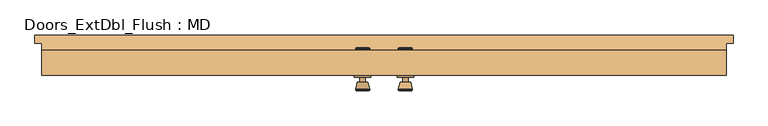
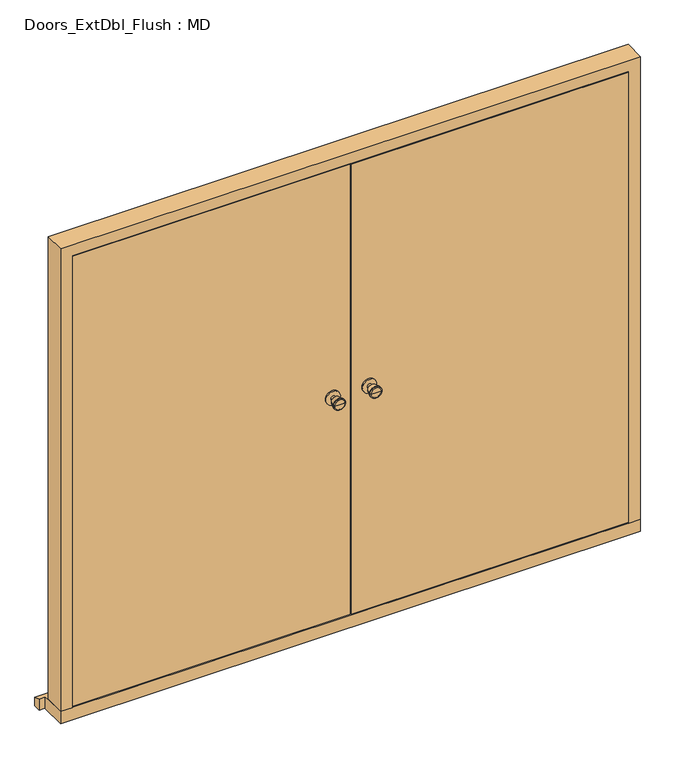
"""IFC4 building model written with IfcOpenShell, lengths in millimetres: door geometry, Doors_ExtDbl_Flush : MD."""

from ifc_helpers import new_model, si_unit, point, frame, frame_2d, origin, place, context, project, spatial, polyline, circle_curve, trimmed, segment, composite_curve, outline, extrude, faceted_brep, source, transform, mapped, element, save
from ifc_brep_helpers import plane_surface, cylinder_surface, revolved_surface, advanced_brep


def doors_extdbl_flush_md_0ef74d11(model_context):
    return source(origin(), model_context, "Body", "SolidModel", [
        advanced_brep(
        [(-76.5, -5.7, 1050.0), (-66.5, -5.7, 1050.0), (-86.5, -5.7, 1050.0), (-96.9758676, -54.7, 1050.0), (-56.0241324, -54.7, 1050.0), (-76.5, -54.7, 1050.0), (-101.5, -52.8721319, 1050.0), (-51.5, -52.8721319, 1050.0), (-101.5, -49.4084537, 1050.0), (-51.5, -49.4084537, 1050.0), (-95.136236, -24.7, 1050.0), (-57.863764, -24.7, 1050.0), (-86.5, -24.7, 1050.0), (-66.5, -24.7, 1050.0)],
        [
            (0, 1),
            (1, 2, circle_curve(frame((-76.5, -5.7, 1050.0), z_axis=(0.0, 1.0, 0.0), x_axis=(1.0, 0.0, 0.0)), 10.0)),
            (2, 0),
            (2, 1, circle_curve(frame((-76.5, -5.7, 1050.0), z_axis=(0.0, 1.0, 0.0), x_axis=(1.0, 0.0, 0.0)), 10.0)),
            (3, 4, circle_curve(frame((-76.5, -54.7, 1050.0), z_axis=(0.0, -1.0, 0.0), x_axis=(1.0, 0.0, 0.0)), 20.4758676)),
            (4, 5),
            (5, 3),
            (4, 3, circle_curve(frame((-76.5, -54.7, 1050.0), z_axis=(0.0, -1.0, 0.0), x_axis=(1.0, 0.0, 0.0)), 20.4758676)),
            (6, 7, circle_curve(frame((-76.5, -52.8721319, 1050.0), z_axis=(0.0, -1.0, 0.0), x_axis=(1.0, 0.0, 0.0)), 25.0)),
            (7, 4),
            (3, 6),
            (7, 6, circle_curve(frame((-76.5, -52.8721319, 1050.0), z_axis=(0.0, -1.0, 0.0), x_axis=(1.0, 0.0, 0.0)), 25.0)),
            (8, 9, circle_curve(frame((-76.5, -49.4084537, 1050.0), z_axis=(0.0, -1.0, 0.0), x_axis=(1.0, 0.0, 0.0)), 25.0)),
            (9, 7),
            (6, 8),
            (9, 8, circle_curve(frame((-76.5, -49.4084537, 1050.0), z_axis=(0.0, -1.0, 0.0), x_axis=(1.0, 0.0, 0.0)), 25.0)),
            (10, 11, circle_curve(frame((-76.5, -24.7, 1050.0), z_axis=(0.0, -1.0, 0.0), x_axis=(1.0, 0.0, 0.0)), 18.636236)),
            (11, 9),
            (8, 10),
            (11, 10, circle_curve(frame((-76.5, -24.7, 1050.0), z_axis=(0.0, -1.0, 0.0), x_axis=(1.0, 0.0, 0.0)), 18.636236)),
            (12, 13, circle_curve(frame((-76.5, -24.7, 1050.0), z_axis=(0.0, -1.0, 0.0), x_axis=(1.0, 0.0, 0.0)), 10.0)),
            (13, 11),
            (10, 12),
            (13, 12, circle_curve(frame((-76.5, -24.7, 1050.0), z_axis=(0.0, -1.0, 0.0), x_axis=(1.0, 0.0, 0.0)), 10.0)),
            (1, 13),
            (12, 2),
        ],
        [
            plane_surface(frame((-76.5, -5.7, 1050.0), z_axis=(0.0, 1.0, 0.0), x_axis=(1.0, 0.0, 0.0))),
            plane_surface(frame((-76.5, -54.7, 1050.0), z_axis=(0.0, -1.0, 0.0), x_axis=(1.0, 0.0, 0.0))),
            revolved_surface(polyline([(-56.0241324, -54.7, 1050.0), (-51.5, -52.8721319, 1050.0)]), (-76.5, -5.7, 1050.0), (0.0, 1.0, 0.0)),
            cylinder_surface(frame((-76.5, -5.7, 1050.0), z_axis=(0.0, 1.0, 0.0), x_axis=(1.0, 0.0, 0.0)), 25.0),
            revolved_surface(polyline([(-51.5, -49.4084537, 1050.0), (-57.863764, -24.7, 1050.0)]), (-76.5, -5.7, 1050.0), (0.0, 1.0, 0.0)),
            plane_surface(frame((-76.5, -24.7, 1050.0), z_axis=(0.0, 1.0, 0.0), x_axis=(1.0, 0.0, 0.0))),
            cylinder_surface(frame((-76.5, -5.7, 1050.0), z_axis=(0.0, 1.0, 0.0), x_axis=(1.0, 0.0, 0.0)), 10.0),
        ],
        [
            (0, [[1, 2, 3]]),
            (0, [[-3, 4, -1]]),
            (1, [[5, 6, 7]]),
            (1, [[8, -7, -6]]),
            (2, [[9, 10, -5, 11]]),
            (2, [[12, -11, -8, -10]]),
            (3, [[13, 14, -9, 15]]),
            (3, [[16, -15, -12, -14]]),
            (4, [[17, 18, -13, 19]]),
            (4, [[20, -19, -16, -18]]),
            (5, [[21, 22, -17, 23]]),
            (5, [[24, -23, -20, -22]]),
            (6, [[-2, 25, -21, 26]]),
            (6, [[-4, -26, -24, -25]]),
        ],
    ),
        extrude(outline(composite_curve([segment(trimmed(circle_curve(frame_2d((1050.0, -76.5)), 30.0), [point((1050.0, -46.5))], [point((1050.0, -106.5))], False, "CARTESIAN"), True, "CONTINUOUS"), segment(trimmed(circle_curve(frame_2d((1050.0, -76.5)), 30.0), [point((1050.0, -106.5))], [point((1050.0, -46.5))], False, "CARTESIAN"), True, "CONTINUOUS")], self_intersect=False)), frame((0.0, -5.7, 0.0), z_axis=(0.0, 1.0, 0.0), x_axis=(0.0, 0.0, 1.0)), (0.0, 0.0, 1.0), 6.0),
        advanced_brep(
        [(-76.5, 50.3, 1050.0), (-86.5, 50.3, 1050.0), (-66.5, 50.3, 1050.0), (-96.9758676, 99.3, 1050.0), (-76.5, 99.3, 1050.0), (-56.0241324, 99.3, 1050.0), (-101.5, 97.4721319, 1050.0), (-51.5, 97.4721319, 1050.0), (-101.5, 94.0084537, 1050.0), (-51.5, 94.0084537, 1050.0), (-95.136236, 69.3, 1050.0), (-57.863764, 69.3, 1050.0), (-86.5, 69.3, 1050.0), (-66.5, 69.3, 1050.0)],
        [
            (0, 1),
            (1, 2, circle_curve(frame((-76.5, 50.3, 1050.0), z_axis=(0.0, -1.0, 0.0), x_axis=(1.0, 0.0, 0.0)), 10.0)),
            (2, 0),
            (2, 1, circle_curve(frame((-76.5, 50.3, 1050.0), z_axis=(0.0, -1.0, 0.0), x_axis=(1.0, 0.0, 0.0)), 10.0)),
            (3, 4),
            (4, 5),
            (5, 3, circle_curve(frame((-76.5, 99.3, 1050.0), z_axis=(0.0, 1.0, 0.0), x_axis=(1.0, 0.0, 0.0)), 20.4758676)),
            (3, 5, circle_curve(frame((-76.5, 99.3, 1050.0), z_axis=(0.0, 1.0, 0.0), x_axis=(1.0, 0.0, 0.0)), 20.4758676)),
            (6, 3),
            (5, 7),
            (7, 6, circle_curve(frame((-76.5, 97.4721319, 1050.0), z_axis=(0.0, 1.0, 0.0), x_axis=(1.0, 0.0, 0.0)), 25.0)),
            (6, 7, circle_curve(frame((-76.5, 97.4721319, 1050.0), z_axis=(0.0, 1.0, 0.0), x_axis=(1.0, 0.0, 0.0)), 25.0)),
            (8, 6),
            (7, 9),
            (9, 8, circle_curve(frame((-76.5, 94.0084537, 1050.0), z_axis=(0.0, 1.0, 0.0), x_axis=(1.0, 0.0, 0.0)), 25.0)),
            (8, 9, circle_curve(frame((-76.5, 94.0084537, 1050.0), z_axis=(0.0, 1.0, 0.0), x_axis=(1.0, 0.0, 0.0)), 25.0)),
            (10, 8),
            (9, 11),
            (11, 10, circle_curve(frame((-76.5, 69.3, 1050.0), z_axis=(0.0, 1.0, 0.0), x_axis=(1.0, 0.0, 0.0)), 18.636236)),
            (10, 11, circle_curve(frame((-76.5, 69.3, 1050.0), z_axis=(0.0, 1.0, 0.0), x_axis=(1.0, 0.0, 0.0)), 18.636236)),
            (12, 10),
            (11, 13),
            (13, 12, circle_curve(frame((-76.5, 69.3, 1050.0), z_axis=(0.0, 1.0, 0.0), x_axis=(1.0, 0.0, 0.0)), 10.0)),
            (12, 13, circle_curve(frame((-76.5, 69.3, 1050.0), z_axis=(0.0, 1.0, 0.0), x_axis=(1.0, 0.0, 0.0)), 10.0)),
            (1, 12),
            (13, 2),
        ],
        [
            plane_surface(frame((-76.5, 50.3, 1050.0), z_axis=(0.0, -1.0, 0.0), x_axis=(1.0, 0.0, 0.0))),
            plane_surface(frame((-76.5, 99.3, 1050.0), z_axis=(0.0, 1.0, 0.0), x_axis=(1.0, 0.0, 0.0))),
            revolved_surface(polyline([(-56.0241324, 99.3, 1050.0), (-51.5, 97.4721319, 1050.0)]), (-76.5, 50.3, 1050.0), (0.0, -1.0, 0.0)),
            cylinder_surface(frame((-76.5, 50.3, 1050.0), z_axis=(0.0, -1.0, 0.0), x_axis=(1.0, 0.0, 0.0)), 25.0),
            revolved_surface(polyline([(-51.5, 94.0084537, 1050.0), (-57.863764, 69.3, 1050.0)]), (-76.5, 50.3, 1050.0), (0.0, -1.0, 0.0)),
            plane_surface(frame((-76.5, 69.3, 1050.0), z_axis=(0.0, -1.0, 0.0), x_axis=(1.0, 0.0, 0.0))),
            cylinder_surface(frame((-76.5, 50.3, 1050.0), z_axis=(0.0, -1.0, 0.0), x_axis=(1.0, 0.0, 0.0)), 10.0),
        ],
        [
            (0, [[1, 2, 3]]),
            (0, [[-3, 4, -1]]),
            (1, [[5, 6, 7]]),
            (1, [[-6, -5, 8]]),
            (2, [[9, -7, 10, 11]]),
            (2, [[-10, -8, -9, 12]]),
            (3, [[13, -11, 14, 15]]),
            (3, [[-14, -12, -13, 16]]),
            (4, [[17, -15, 18, 19]]),
            (4, [[-18, -16, -17, 20]]),
            (5, [[21, -19, 22, 23]]),
            (5, [[-22, -20, -21, 24]]),
            (6, [[25, -23, 26, -2]]),
            (6, [[-26, -24, -25, -4]]),
        ],
    ),
        extrude(outline(composite_curve([segment(trimmed(circle_curve(frame_2d((1050.0, -76.5)), 30.0), [point((1050.0, -46.5))], [point((1050.0, -106.5))], False, "CARTESIAN"), True, "CONTINUOUS"), segment(trimmed(circle_curve(frame_2d((1050.0, -76.5)), 30.0), [point((1050.0, -106.5))], [point((1050.0, -46.5))], False, "CARTESIAN"), True, "CONTINUOUS")], self_intersect=False)), frame((0.0, 44.3, 0.0), z_axis=(0.0, 1.0, 0.0), x_axis=(0.0, 0.0, 1.0)), (0.0, 0.0, 1.0), 6.0),
        advanced_brep(
        [(76.5, -5.7, 1050.0), (86.5, -5.7, 1050.0), (66.5, -5.7, 1050.0), (96.9758676, -54.7, 1050.0), (76.5, -54.7, 1050.0), (56.0241324, -54.7, 1050.0), (101.5, -52.8721319, 1050.0), (51.5, -52.8721319, 1050.0), (101.5, -49.4084537, 1050.0), (51.5, -49.4084537, 1050.0), (95.136236, -24.7, 1050.0), (57.863764, -24.7, 1050.0), (86.5, -24.7, 1050.0), (66.5, -24.7, 1050.0)],
        [
            (0, 1),
            (1, 2, circle_curve(frame((76.5, -5.7, 1050.0), z_axis=(0.0, 1.0, 0.0), x_axis=(-1.0, 0.0, 0.0)), 10.0)),
            (2, 0),
            (2, 1, circle_curve(frame((76.5, -5.7, 1050.0), z_axis=(0.0, 1.0, 0.0), x_axis=(-1.0, 0.0, 0.0)), 10.0)),
            (3, 4),
            (4, 5),
            (5, 3, circle_curve(frame((76.5, -54.7, 1050.0), z_axis=(0.0, -1.0, 0.0), x_axis=(-1.0, 0.0, 0.0)), 20.4758676)),
            (3, 5, circle_curve(frame((76.5, -54.7, 1050.0), z_axis=(0.0, -1.0, 0.0), x_axis=(-1.0, 0.0, 0.0)), 20.4758676)),
            (6, 3),
            (5, 7),
            (7, 6, circle_curve(frame((76.5, -52.8721319, 1050.0), z_axis=(0.0, -1.0, 0.0), x_axis=(-1.0, 0.0, 0.0)), 25.0)),
            (6, 7, circle_curve(frame((76.5, -52.8721319, 1050.0), z_axis=(0.0, -1.0, 0.0), x_axis=(-1.0, 0.0, 0.0)), 25.0)),
            (8, 6),
            (7, 9),
            (9, 8, circle_curve(frame((76.5, -49.4084537, 1050.0), z_axis=(0.0, -1.0, 0.0), x_axis=(-1.0, 0.0, 0.0)), 25.0)),
            (8, 9, circle_curve(frame((76.5, -49.4084537, 1050.0), z_axis=(0.0, -1.0, 0.0), x_axis=(-1.0, 0.0, 0.0)), 25.0)),
            (10, 8),
            (9, 11),
            (11, 10, circle_curve(frame((76.5, -24.7, 1050.0), z_axis=(0.0, -1.0, 0.0), x_axis=(-1.0, 0.0, 0.0)), 18.636236)),
            (10, 11, circle_curve(frame((76.5, -24.7, 1050.0), z_axis=(0.0, -1.0, 0.0), x_axis=(-1.0, 0.0, 0.0)), 18.636236)),
            (12, 10),
            (11, 13),
            (13, 12, circle_curve(frame((76.5, -24.7, 1050.0), z_axis=(0.0, -1.0, 0.0), x_axis=(-1.0, 0.0, 0.0)), 10.0)),
            (12, 13, circle_curve(frame((76.5, -24.7, 1050.0), z_axis=(0.0, -1.0, 0.0), x_axis=(-1.0, 0.0, 0.0)), 10.0)),
            (1, 12),
            (13, 2),
        ],
        [
            plane_surface(frame((76.5, -5.7, 1050.0), z_axis=(0.0, 1.0, 0.0), x_axis=(-1.0, 0.0, 0.0))),
            plane_surface(frame((76.5, -54.7, 1050.0), z_axis=(0.0, -1.0, 0.0), x_axis=(-1.0, 0.0, 0.0))),
            revolved_surface(polyline([(56.0241324, -54.7, 1050.0), (51.5, -52.8721319, 1050.0)]), (76.5, -5.7, 1050.0), (0.0, 1.0, 0.0)),
            cylinder_surface(frame((76.5, -5.7, 1050.0), z_axis=(0.0, 1.0, 0.0), x_axis=(-1.0, 0.0, 0.0)), 25.0),
            revolved_surface(polyline([(51.5, -49.4084537, 1050.0), (57.863764, -24.7, 1050.0)]), (76.5, -5.7, 1050.0), (0.0, 1.0, 0.0)),
            plane_surface(frame((76.5, -24.7, 1050.0), z_axis=(0.0, 1.0, 0.0), x_axis=(-1.0, 0.0, 0.0))),
            cylinder_surface(frame((76.5, -5.7, 1050.0), z_axis=(0.0, 1.0, 0.0), x_axis=(-1.0, 0.0, 0.0)), 10.0),
        ],
        [
            (0, [[1, 2, 3]]),
            (0, [[-3, 4, -1]]),
            (1, [[5, 6, 7]]),
            (1, [[-6, -5, 8]]),
            (2, [[9, -7, 10, 11]]),
            (2, [[-10, -8, -9, 12]]),
            (3, [[13, -11, 14, 15]]),
            (3, [[-14, -12, -13, 16]]),
            (4, [[17, -15, 18, 19]]),
            (4, [[-18, -16, -17, 20]]),
            (5, [[21, -19, 22, 23]]),
            (5, [[-22, -20, -21, 24]]),
            (6, [[25, -23, 26, -2]]),
            (6, [[-26, -24, -25, -4]]),
        ],
    ),
        extrude(outline(composite_curve([segment(trimmed(circle_curve(frame_2d((1050.0, 76.5)), 30.0), [point((1050.0, 46.5))], [point((1050.0, 106.5))], False, "CARTESIAN"), True, "CONTINUOUS"), segment(trimmed(circle_curve(frame_2d((1050.0, 76.5)), 30.0), [point((1050.0, 106.5))], [point((1050.0, 46.5))], False, "CARTESIAN"), True, "CONTINUOUS")], self_intersect=False)), frame((0.0, -5.7, 0.0), z_axis=(0.0, 1.0, 0.0), x_axis=(0.0, 0.0, 1.0)), (0.0, 0.0, 1.0), 6.0),
        advanced_brep(
        [(76.5, 50.3, 1050.0), (66.5, 50.3, 1050.0), (86.5, 50.3, 1050.0), (96.9758676, 99.3, 1050.0), (56.0241324, 99.3, 1050.0), (76.5, 99.3, 1050.0), (101.5, 97.4721319, 1050.0), (51.5, 97.4721319, 1050.0), (101.5, 94.0084537, 1050.0), (51.5, 94.0084537, 1050.0), (95.136236, 69.3, 1050.0), (57.863764, 69.3, 1050.0), (86.5, 69.3, 1050.0), (66.5, 69.3, 1050.0)],
        [
            (0, 1),
            (1, 2, circle_curve(frame((76.5, 50.3, 1050.0), z_axis=(0.0, -1.0, 0.0), x_axis=(-1.0, 0.0, 0.0)), 10.0)),
            (2, 0),
            (2, 1, circle_curve(frame((76.5, 50.3, 1050.0), z_axis=(0.0, -1.0, 0.0), x_axis=(-1.0, 0.0, 0.0)), 10.0)),
            (3, 4, circle_curve(frame((76.5, 99.3, 1050.0), z_axis=(0.0, 1.0, 0.0), x_axis=(-1.0, 0.0, 0.0)), 20.4758676)),
            (4, 5),
            (5, 3),
            (4, 3, circle_curve(frame((76.5, 99.3, 1050.0), z_axis=(0.0, 1.0, 0.0), x_axis=(-1.0, 0.0, 0.0)), 20.4758676)),
            (6, 7, circle_curve(frame((76.5, 97.4721319, 1050.0), z_axis=(0.0, 1.0, 0.0), x_axis=(-1.0, 0.0, 0.0)), 25.0)),
            (7, 4),
            (3, 6),
            (7, 6, circle_curve(frame((76.5, 97.4721319, 1050.0), z_axis=(0.0, 1.0, 0.0), x_axis=(-1.0, 0.0, 0.0)), 25.0)),
            (8, 9, circle_curve(frame((76.5, 94.0084537, 1050.0), z_axis=(0.0, 1.0, 0.0), x_axis=(-1.0, 0.0, 0.0)), 25.0)),
            (9, 7),
            (6, 8),
            (9, 8, circle_curve(frame((76.5, 94.0084537, 1050.0), z_axis=(0.0, 1.0, 0.0), x_axis=(-1.0, 0.0, 0.0)), 25.0)),
            (10, 11, circle_curve(frame((76.5, 69.3, 1050.0), z_axis=(0.0, 1.0, 0.0), x_axis=(-1.0, 0.0, 0.0)), 18.636236)),
            (11, 9),
            (8, 10),
            (11, 10, circle_curve(frame((76.5, 69.3, 1050.0), z_axis=(0.0, 1.0, 0.0), x_axis=(-1.0, 0.0, 0.0)), 18.636236)),
            (12, 13, circle_curve(frame((76.5, 69.3, 1050.0), z_axis=(0.0, 1.0, 0.0), x_axis=(-1.0, 0.0, 0.0)), 10.0)),
            (13, 11),
            (10, 12),
            (13, 12, circle_curve(frame((76.5, 69.3, 1050.0), z_axis=(0.0, 1.0, 0.0), x_axis=(-1.0, 0.0, 0.0)), 10.0)),
            (1, 13),
            (12, 2),
        ],
        [
            plane_surface(frame((76.5, 50.3, 1050.0), z_axis=(0.0, -1.0, 0.0), x_axis=(-1.0, 0.0, 0.0))),
            plane_surface(frame((76.5, 99.3, 1050.0), z_axis=(0.0, 1.0, 0.0), x_axis=(-1.0, 0.0, 0.0))),
            revolved_surface(polyline([(56.0241324, 99.3, 1050.0), (51.5, 97.4721319, 1050.0)]), (76.5, 50.3, 1050.0), (0.0, -1.0, 0.0)),
            cylinder_surface(frame((76.5, 50.3, 1050.0), z_axis=(0.0, -1.0, 0.0), x_axis=(-1.0, 0.0, 0.0)), 25.0),
            revolved_surface(polyline([(51.5, 94.0084537, 1050.0), (57.863764, 69.3, 1050.0)]), (76.5, 50.3, 1050.0), (0.0, -1.0, 0.0)),
            plane_surface(frame((76.5, 69.3, 1050.0), z_axis=(0.0, -1.0, 0.0), x_axis=(-1.0, 0.0, 0.0))),
            cylinder_surface(frame((76.5, 50.3, 1050.0), z_axis=(0.0, -1.0, 0.0), x_axis=(-1.0, 0.0, 0.0)), 10.0),
        ],
        [
            (0, [[1, 2, 3]]),
            (0, [[-3, 4, -1]]),
            (1, [[5, 6, 7]]),
            (1, [[8, -7, -6]]),
            (2, [[9, 10, -5, 11]]),
            (2, [[12, -11, -8, -10]]),
            (3, [[13, 14, -9, 15]]),
            (3, [[16, -15, -12, -14]]),
            (4, [[17, 18, -13, 19]]),
            (4, [[20, -19, -16, -18]]),
            (5, [[21, 22, -17, 23]]),
            (5, [[24, -23, -20, -22]]),
            (6, [[-2, 25, -21, 26]]),
            (6, [[-4, -26, -24, -25]]),
        ],
    ),
        extrude(outline(composite_curve([segment(trimmed(circle_curve(frame_2d((1050.0, 76.5)), 30.0), [point((1050.0, 46.5))], [point((1050.0, 106.5))], False, "CARTESIAN"), True, "CONTINUOUS"), segment(trimmed(circle_curve(frame_2d((1050.0, 76.5)), 30.0), [point((1050.0, 106.5))], [point((1050.0, 46.5))], False, "CARTESIAN"), True, "CONTINUOUS")], self_intersect=False)), frame((0.0, 44.3, 0.0), z_axis=(0.0, 1.0, 0.0), x_axis=(0.0, 0.0, 1.0)), (0.0, 0.0, 1.0), 6.0),
        faceted_brep([(1148.7, 89.3, 54.5), (1219.2, 89.3, 54.5), (1219.2, 0.3, 54.5), (1170.7, 0.3, 54.5), (1170.7, 47.3, 54.5), (1148.7, 47.3, 54.5), (1148.7, 89.3, 2039.5), (-1148.7, 89.3, 2039.5), (-1148.7, 89.3, 54.5), (-1219.2, 89.3, 54.5), (-1219.2, 89.3, 2110.0), (1219.2, 89.3, 2110.0), (1219.2, 0.3, 2110.0), (-1219.2, 0.3, 2110.0), (-1219.2, 0.3, 54.5), (-1170.7, 0.3, 54.5), (-1170.7, 0.3, 2061.5), (1170.7, 0.3, 2061.5), (1170.7, 47.3, 2061.5), (-1170.7, 47.3, 2061.5), (-1170.7, 47.3, 54.5), (-1148.7, 47.3, 54.5), (-1148.7, 47.3, 2039.5), (1148.7, 47.3, 2039.5)], [[[0, 1, 2, 3, 4, 5]], [[1, 0, 6, 7, 8, 9, 10, 11]], [[2, 1, 11, 12]], [[3, 2, 12, 13, 14, 15, 16, 17]], [[4, 3, 17, 18]], [[5, 4, 18, 19, 20, 21, 22, 23]], [[0, 5, 23, 6]], [[7, 22, 21, 8]], [[8, 21, 20, 15, 14, 9]], [[13, 10, 9, 14]], [[19, 16, 15, 20]], [[12, 11, 10, 13]], [[18, 17, 16, 19]], [[6, 23, 22, 7]]]),
        faceted_brep([(1244.2, 144.3, 0.0), (1244.2, 144.3, 38.5947221), (1244.2, 114.3, 47.2703282), (1244.2, 114.3, 0.0), (-1244.2, 144.3, 38.5947221), (-1244.2, 144.3, 0.0), (-1244.2, 114.3, 0.0), (-1244.2, 114.3, 47.2703282), (1219.2, 114.3, 0.0), (1219.2, 0.3, 0.0), (-1219.2, 0.3, 0.0), (-1219.2, 114.3, 0.0), (-1219.2, 114.3, 47.2703282), (-1219.2, 89.3, 54.5), (1219.2, 89.3, 54.5), (1219.2, 114.3, 47.2703282), (-1219.2, 0.3, 54.5), (1219.2, 0.3, 54.5)], [[[0, 1, 2, 3]], [[4, 5, 6, 7]], [[5, 0, 3, 8, 9, 10, 11, 6]], [[1, 0, 5, 4]], [[1, 4, 7, 12, 13, 14, 15, 2]], [[13, 16, 17, 14]], [[16, 10, 9, 17]], [[12, 11, 10, 16, 13]], [[11, 12, 7, 6]], [[8, 15, 14, 17, 9]], [[15, 8, 3, 2]]]),
        extrude(outline(polyline([(1167.7, 0.3), (1.5, 0.3), (1.5, 44.3), (1167.7, 44.3), (1167.7, 0.3)])), frame((0.0, 0.0, 58.5), z_axis=(0.0, 0.0, 1.0), x_axis=(1.0, 0.0, 0.0)), (0.0, 0.0, 1.0), 2000.0),
        extrude(outline(polyline([(-1.5, 0.3), (-1167.7, 0.3), (-1167.7, 44.3), (-1.5, 44.3), (-1.5, 0.3)])), frame((0.0, 0.0, 58.5), z_axis=(0.0, 0.0, 1.0), x_axis=(1.0, 0.0, 0.0)), (0.0, 0.0, 1.0), 2000.0),
    ])


if __name__ == "__main__":
    model = new_model("IFC4")
    model_context = context("Model", 3, world=origin())
    ifc_project = project(units=[si_unit("LENGTHUNIT", "METRE", prefix="MILLI")], contexts=[model_context])
    site = spatial("IfcSite", under=ifc_project)
    building = spatial("IfcBuilding", under=site)
    placement = place(None, origin())
    doors_extdbl_flush_md_shape = doors_extdbl_flush_md_0ef74d11(model_context)
    element("IfcDoor", 1, ObjectType="Doors_ExtDbl_Flush : MD", at=placement, inside=building, context=model_context, shape_type="MappedRepresentation", body=[
        mapped(doors_extdbl_flush_md_shape, transform((0.0, 0.0, 0.0), x_axis=(1.0, 0.0, 0.0), y_axis=(0.0, 1.0, 0.0), z_axis=(0.0, 0.0, 1.0))),
    ])
    save(model, "model.ifc")

# Revit data of these elements
# Type "Doors_ExtDbl_Flush : MD"
#   Type Mark = "47"
#   Type Comments = "External Double"
#   Operation = "DoubleDoorSingleSwing"
#   Keynote = "L20"
#   Analytic Construction = "Metal"
#   Wrap Layers (Ext) from Ext = 0' - 4.03543"
#   Wrap Layers (Int) from Ext = 0' - 6.98819"
#   Thickness = 0' - 1.73228"
#   Rough Width = 8' - 0"
#   Rough Height = 6' - 11.07087"
#   O/A Frame Width = 0' - 2.51969"
#   Heat Transfer Coefficient (U) = 3.7021 W/(m²·K)
#   Handle Z Distance = 3' - 5.33858"
#   FrameWidth = 0' - 1.65354"
#   FrameOffset - External = 0' - 0.98425"
#   FrameDepth = 0' - 3.50394"
#   Door Panel Width = 3' - 9.91339"
#   Door Panel Thickness = 0' - 1.73228"
#   Door Panel Height = 6' - 6.74016"
#   Cill Thickness = 0' - 2.14567"
#   Cill Projection = 0' - 1.1811"
#   Handle X Distance = 0' - 2.95276"
#   Height = 6' - 11.07087"
#   Structural Tolerance = 0' - 0.25591"
#   Tolerance = 0' - 0.11811"
#   Undercut = 0' - 0.15748"
#   Width = 8' - 0"
#   Cill Extension = 0' - 0.98425"
#   Cavity Closer Width = 0' - 1.9685"
#   Cavity Closer Offset from Ext = 0' - 4.03543"
#   Cavity Closer Depth = 0' - 3.34646"
#   Vis - Ironmongery = yes
#   Vis - Cavity Closers = yes
#   Function = 1
#   Material Door = Door - Panel
#   Material Frame = Door - Frame/Mullion
#   Material Ironmongery = Door - Handle
#   Visual Light Transmittance = 0
#   Thermal Resistance (R) = 0
#   Solar Heat Gain Coefficient = 0
#   Wall Closure = (empty or 0)
# Element 1 (IfcDoor, "Doors_ExtDbl_Flush : MD")
#   Materials on its faces: "Door - Handle", "Door - Frame/Mullion", "Door - Panel"
# Materials
#   "Door - Panel": class "Wood", colour RGB 210 159 95, transparency 0, Keynote = "L20", Cost = 0
#   "Door - Frame/Mullion": class "Wood", colour RGB 212 179 113, transparency 0, Keynote = "L20", Cost = 0
#   "Door - Handle": colour RGB 0 0 0, transparency 0, Keynote = "P21", Cost = 0
